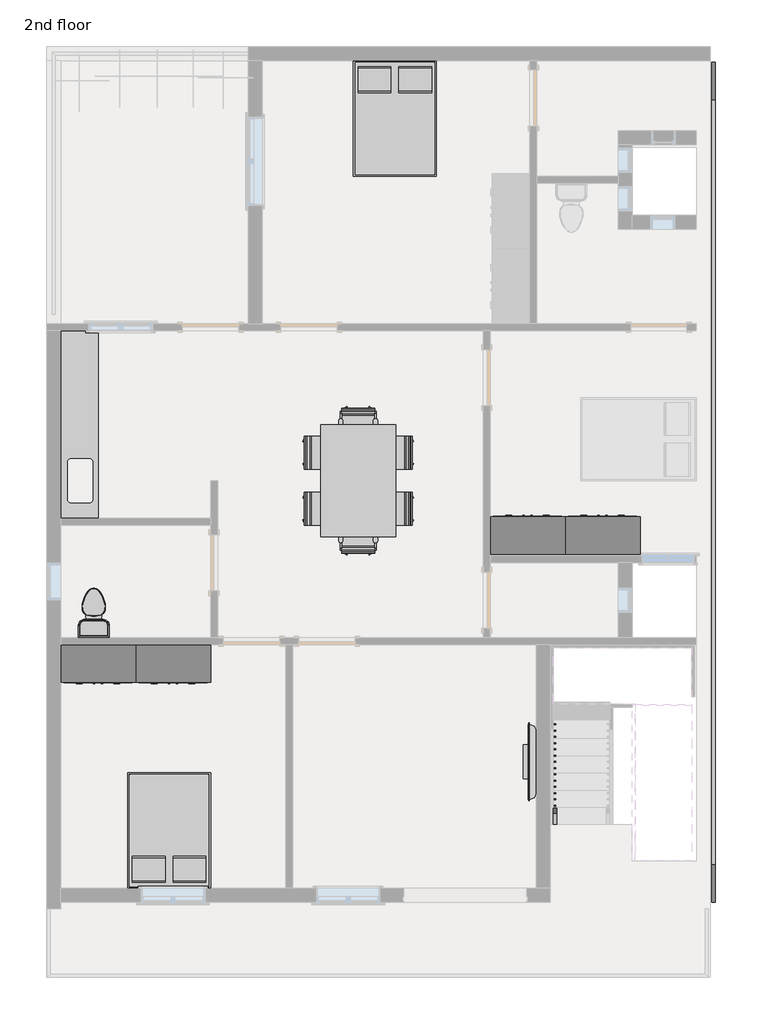
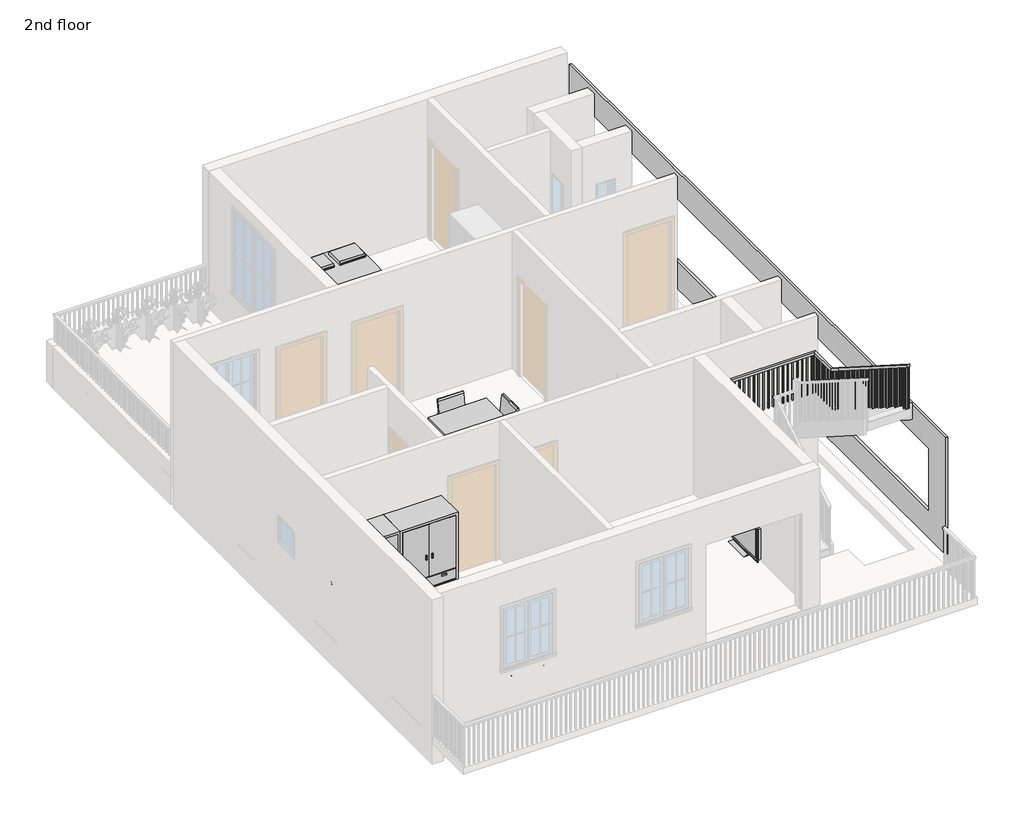
# One storey, part 4 of 5: 16 furniture elements, 1 flow terminal, 1 railing.
"""IFC4 building model written with IfcOpenShell, lengths in millimetres."""

from ifc_helpers import new_model, si_unit, frame, origin, place, context, project, spatial, polyline, outline, extrude, faceted_brep, transform, mapped, element, save
from components import toilet_domestic_3d_toilet_domestic_3d_9ecb9d01, toilet_domestic_3d_toilet_domestic_3d_e67c3c64, furniture_b58f7881, casework_4_casework_4_12d1038f, chair_task_chair_task_b7f3823b, chair_task_arms_chair_task_arms_fa5a08ef, furniture_771c7099, furniture_0b81fedb, furniture_0bcc43ae, furniture_82e269c4

model = new_model("IFC4")

# Units and contexts
model_context = context("Model", 3, world=origin())
ifc_project = project(units=[si_unit("LENGTHUNIT", "METRE", prefix="MILLI")], contexts=[model_context])

# Site, building, storey
site = spatial("IfcSite", under=ifc_project)
building = spatial("IfcBuilding", under=site)
storey = spatial("IfcBuildingStorey", under=building, Name="2nd floor", Elevation=7010.4)

# Flow terminal
placement = place(None, origin())
toilet_domestic_3d_toilet_domestic_3d_shape = toilet_domestic_3d_toilet_domestic_3d_9ecb9d01(model_context)
toilet_domestic_3d_toilet_domestic_3d_2_shape = toilet_domestic_3d_toilet_domestic_3d_e67c3c64(model_context)
element("IfcFlowTerminal", 1, ObjectType="Toilet-Domestic-3D : Toilet-Domestic-3D", at=placement, inside=storey, context=model_context, shape_type="MappedRepresentation", body=[
    mapped(toilet_domestic_3d_toilet_domestic_3d_shape, transform((-7342.9058187, 3694.2738062, 7010.4), x_axis=(1.0, 0.0, 0.0), y_axis=(0.0, 1.0, 0.0), z_axis=(0.0, 0.0, 1.0))),
    mapped(toilet_domestic_3d_toilet_domestic_3d_2_shape, transform((-7342.9058187, 3694.2738062, 7010.4), x_axis=(1.0, 0.0, 0.0), y_axis=(0.0, 1.0, 0.0), z_axis=(0.0, 0.0, 1.0))),
])

# Furniture
furniture_shape = furniture_b58f7881(model_context)
element("IfcFurniture", 2, ObjectType="Bed-Box : Double 53\" x 74\"", at=placement, inside=storey, context=model_context, shape_type="MappedRepresentation", body=[
    mapped(furniture_shape, transform((-2785.3023187, 11872.8553007, 7010.4), x_axis=(1.0, 0.0, 0.0), y_axis=(0.0, 1.0, 0.0), z_axis=(0.0, 0.0, 1.0))),
])
element("IfcFurniture", 3, ObjectType="Bed-Box : Double 53\" x 74\"", at=placement, inside=storey, context=model_context, shape_type="MappedRepresentation", body=[
    mapped(furniture_shape, transform((-5777.2974007, -178.4037157, 7010.4), x_axis=(-1.0, 0.0, 0.0), y_axis=(0.0, -1.0, 0.0), z_axis=(0.0, 0.0, 1.0))),
])
casework_4_casework_4_shape = casework_4_casework_4_12d1038f(model_context)
element("IfcFurniture", 4, ObjectType="Casework 4 : Casework 4", at=placement, inside=storey, context=model_context, shape_type="MappedRepresentation", body=[
    mapped(casework_4_casework_4_shape, transform((0.0, 0.0, 0.0), x_axis=(1.0, 0.0, 0.0), y_axis=(0.0, 1.0, 0.0), z_axis=(0.0, 0.0, 1.0))),
])
chair_task_chair_task_shape = chair_task_chair_task_b7f3823b(model_context)
element("IfcFurniture", 5, ObjectType="Chair-Task : Chair-Task", at=placement, inside=storey, context=model_context, shape_type="MappedRepresentation", body=[
    mapped(chair_task_chair_task_shape, transform((-3671.5957614, 6343.8166122, 7010.4), x_axis=(0.0, -1.0, 0.0), y_axis=(1.0, 0.0, 0.0), z_axis=(0.0, 0.0, 1.0))),
])
element("IfcFurniture", 6, ObjectType="Chair-Task : Chair-Task", at=placement, inside=storey, context=model_context, shape_type="MappedRepresentation", body=[
    mapped(chair_task_chair_task_shape, transform((-2414.5039581, 6061.8349729, 7010.4), x_axis=(0.0, 1.0, 0.0), y_axis=(-1.0, 0.0, 0.0), z_axis=(0.0, 0.0, 1.0))),
])
element("IfcFurniture", 7, ObjectType="Chair-Task : Chair-Task", at=placement, inside=storey, context=model_context, shape_type="MappedRepresentation", body=[
    mapped(chair_task_chair_task_shape, transform((-3671.5957614, 5429.4166122, 7010.4), x_axis=(0.0, -1.0, 0.0), y_axis=(1.0, 0.0, 0.0), z_axis=(0.0, 0.0, 1.0))),
])
element("IfcFurniture", 8, ObjectType="Chair-Task : Chair-Task", at=placement, inside=storey, context=model_context, shape_type="MappedRepresentation", body=[
    mapped(chair_task_chair_task_shape, transform((-2414.5039581, 5147.4349729, 7010.4), x_axis=(0.0, 1.0, 0.0), y_axis=(-1.0, 0.0, 0.0), z_axis=(0.0, 0.0, 1.0))),
])
chair_task_arms_chair_task_arms_shape = chair_task_arms_chair_task_arms_fa5a08ef(model_context)
element("IfcFurniture", 9, ObjectType="Chair-Task Arms : Chair-Task Arms", at=placement, inside=storey, context=model_context, shape_type="MappedRepresentation", body=[
    mapped(chair_task_arms_chair_task_arms_shape, transform((-3184.0406794, 4812.2798909, 7010.4), x_axis=(1.0, 0.0, 0.0), y_axis=(0.0, 1.0, 0.0), z_axis=(0.0, 0.0, 1.0))),
])
element("IfcFurniture", 10, ObjectType="Chair-Task Arms : Chair-Task Arms", at=placement, inside=storey, context=model_context, shape_type="MappedRepresentation", body=[
    mapped(chair_task_arms_chair_task_arms_shape, transform((-2902.05904, 6678.9716942, 7010.4), x_axis=(-1.0, 0.0, 0.0), y_axis=(0.0, -1.0, 0.0), z_axis=(0.0, 0.0, 1.0))),
])
furniture_2_shape = furniture_771c7099(model_context)
element("IfcFurniture", 11, ObjectType="Counter Top w Sink Hole : 24\" Depth", at=placement, inside=storey, context=model_context, shape_type="MappedRepresentation", body=[
    mapped(furniture_2_shape, transform((-7907.1498597, 6336.4880876, 7010.4), x_axis=(0.0, 1.0, 0.0), y_axis=(-1.0, 0.0, 0.0), z_axis=(0.0, 0.0, 1.0))),
])
furniture_3_shape = furniture_0b81fedb(model_context)
element("IfcFurniture", 12, ObjectType="TV - Flat Screen : 50\"", at=placement, inside=storey, context=model_context, shape_type="MappedRepresentation", body=[
    mapped(furniture_3_shape, transform((-205.9884834, 1169.6812784, 7010.4), x_axis=(0.0, -1.0, 0.0), y_axis=(1.0, 0.0, 0.0), z_axis=(0.0, 0.0, 1.0))),
])
furniture_4_shape = furniture_0bcc43ae(model_context)
element("IfcFurniture", 13, ObjectType="Table-Conference2 w Chairs : 48\" x 144\"", at=placement, inside=storey, context=model_context, shape_type="MappedRepresentation", body=[
    mapped(furniture_4_shape, transform((-3043.0498597, 5745.6257925, 7010.4), x_axis=(0.0, 1.0, 0.0), y_axis=(-1.0, 0.0, 0.0), z_axis=(0.0, 0.0, 1.0))),
])
furniture_5_shape = furniture_82e269c4(model_context)
element("IfcFurniture", 14, ObjectType="Wardrobe : 48\" x 72\" x 24\"", at=placement, inside=storey, context=model_context, shape_type="MappedRepresentation", body=[
    mapped(furniture_5_shape, transform((-556.3431196, 4272.886983, 7010.4), x_axis=(-1.0, 0.0, 0.0), y_axis=(0.0, -1.0, 0.0), z_axis=(0.0, 0.0, 1.0))),
])
element("IfcFurniture", 15, ObjectType="Wardrobe : 48\" x 72\" x 24\"", at=placement, inside=storey, context=model_context, shape_type="MappedRepresentation", body=[
    mapped(furniture_5_shape, transform((662.8568804, 4272.886983, 7010.4), x_axis=(-1.0, 0.0, 0.0), y_axis=(0.0, -1.0, 0.0), z_axis=(0.0, 0.0, 1.0))),
])
element("IfcFurniture", 16, ObjectType="Wardrobe : 48\" x 72\" x 24\"", at=placement, inside=storey, context=model_context, shape_type="MappedRepresentation", body=[
    mapped(furniture_5_shape, transform((-7002.9565999, 3357.5646021, 7010.4), x_axis=(1.0, 0.0, 0.0), y_axis=(0.0, 1.0, 0.0), z_axis=(0.0, 0.0, 1.0))),
])
element("IfcFurniture", 17, ObjectType="Wardrobe : 48\" x 72\" x 24\"", at=placement, inside=storey, context=model_context, shape_type="MappedRepresentation", body=[
    mapped(furniture_5_shape, transform((-5783.7565999, 3357.5646021, 7010.4), x_axis=(1.0, 0.0, 0.0), y_axis=(0.0, 1.0, 0.0), z_axis=(0.0, 0.0, 1.0))),
])

# Railing
element("IfcRailing", 18, ObjectType="Handrail - Rectangular", at=placement, inside=storey, context=model_context, shape_type="SolidModel", body=[
    faceted_brep([(131.9501403, 157.6257925, 8102.6), (131.9501403, 157.6257925, 8042.386276), (182.7501403, 157.6257925, 8042.386276), (182.7501403, 157.6257925, 8102.6), (131.9501403, 2113.4257925, 9347.2), (131.9501403, 2128.2187874, 9296.4), (182.7501403, 2128.2187874, 9296.4), (182.7501403, 2113.4257925, 9347.2), (131.9501403, 3027.8257925, 9347.2), (131.9501403, 3027.8257925, 9296.4), (182.7501403, 2977.0257925, 9296.4), (182.7501403, 2977.0257925, 9347.2), (2379.8501403, 3027.8257925, 9347.2), (2379.8501403, 3027.8257925, 9296.4), (2329.0501403, 2977.0257925, 9296.4), (2329.0501403, 2977.0257925, 9347.2), (2379.8501403, 2392.8257925, 9347.2), (2379.8501403, 2378.0327976, 9296.4), (2329.0501403, 2378.0327976, 9296.4), (2329.0501403, 2392.8257925, 9347.2), (2379.8501403, 2113.4257925, 9525.0), (2379.8501403, 2086.1525175, 9482.1419964), (2329.0501403, 2086.1525175, 9482.1419964), (2329.0501403, 2113.4257925, 9525.0), (2379.8501403, -401.1742075, 11125.2), (2329.0501403, -401.1742075, 11125.2), (2329.0501403, -401.1742075, 11064.986276), (2379.8501403, -401.1742075, 11064.986276)], [[[0, 1, 2, 3]], [[1, 0, 4, 5]], [[2, 1, 5, 6]], [[3, 2, 6, 7]], [[0, 3, 7, 4]], [[5, 4, 8, 9]], [[6, 5, 9, 10]], [[7, 6, 10, 11]], [[4, 7, 11, 8]], [[9, 8, 12, 13]], [[10, 9, 13, 14]], [[11, 10, 14, 15]], [[8, 11, 15, 12]], [[13, 12, 16, 17]], [[14, 13, 17, 18]], [[15, 14, 18, 19]], [[12, 15, 19, 16]], [[17, 16, 20, 21]], [[18, 17, 21, 22]], [[19, 18, 22, 23]], [[16, 19, 23, 20]], [[24, 25, 26, 27]], [[21, 20, 24, 27]], [[22, 21, 27, 26]], [[23, 22, 26, 25]], [[20, 23, 25, 24]]]),
    extrude(outline(polyline([(-315.4492075, 11010.4340032), (-315.4492075, 10033.0), (-334.4992075, 10033.0), (-334.4992075, 11022.5567305), (-315.4492075, 11010.4340032)])), frame((2344.9251403, 0.0, 0.0), z_axis=(1.0, 0.0, 0.0), x_axis=(0.0, 1.0, 0.0)), (0.0, 0.0, 1.0), 19.05),
    extrude(outline(polyline([(-213.8492075, 10945.7794578), (-213.8492075, 10033.0), (-232.8992075, 10033.0), (-232.8992075, 10957.9021851), (-213.8492075, 10945.7794578)])), frame((2344.9251403, 0.0, 0.0), z_axis=(1.0, 0.0, 0.0), x_axis=(0.0, 1.0, 0.0)), (0.0, 0.0, 1.0), 19.05),
    extrude(outline(polyline([(-112.2492075, 10881.1249123), (-112.2492075, 10033.0), (-131.2992075, 10033.0), (-131.2992075, 10893.2476396), (-112.2492075, 10881.1249123)])), frame((2344.9251403, 0.0, 0.0), z_axis=(1.0, 0.0, 0.0), x_axis=(0.0, 1.0, 0.0)), (0.0, 0.0, 1.0), 19.05),
    extrude(outline(polyline([(-10.6492075, 10816.4703669), (-10.6492075, 9855.2), (-29.6992075, 9855.2), (-29.6992075, 10828.5930941), (-10.6492075, 10816.4703669)])), frame((2344.9251403, 0.0, 0.0), z_axis=(1.0, 0.0, 0.0), x_axis=(0.0, 1.0, 0.0)), (0.0, 0.0, 1.0), 19.05),
    extrude(outline(polyline([(90.9507925, 10751.8158214), (90.9507925, 9855.2), (71.9007925, 9855.2), (71.9007925, 10763.9385487), (90.9507925, 10751.8158214)])), frame((2344.9251403, 0.0, 0.0), z_axis=(1.0, 0.0, 0.0), x_axis=(0.0, 1.0, 0.0)), (0.0, 0.0, 1.0), 19.05),
    extrude(outline(polyline([(192.5507925, 10687.161276), (192.5507925, 9677.4), (173.5007925, 9677.4), (173.5007925, 10699.2840032), (192.5507925, 10687.161276)])), frame((2344.9251403, 0.0, 0.0), z_axis=(1.0, 0.0, 0.0), x_axis=(0.0, 1.0, 0.0)), (0.0, 0.0, 1.0), 19.05),
    extrude(outline(polyline([(294.1507925, 10622.5067305), (294.1507925, 9677.4), (275.1007925, 9677.4), (275.1007925, 10634.6294578), (294.1507925, 10622.5067305)])), frame((2344.9251403, 0.0, 0.0), z_axis=(1.0, 0.0, 0.0), x_axis=(0.0, 1.0, 0.0)), (0.0, 0.0, 1.0), 19.05),
    extrude(outline(polyline([(395.7507925, 10557.8521851), (395.7507925, 9677.4), (376.7007925, 9677.4), (376.7007925, 10569.9749123), (395.7507925, 10557.8521851)])), frame((2344.9251403, 0.0, 0.0), z_axis=(1.0, 0.0, 0.0), x_axis=(0.0, 1.0, 0.0)), (0.0, 0.0, 1.0), 19.05),
    extrude(outline(polyline([(497.3507925, 10493.1976396), (497.3507925, 9499.6), (478.3007925, 9499.6), (478.3007925, 10505.3203669), (497.3507925, 10493.1976396)])), frame((2344.9251403, 0.0, 0.0), z_axis=(1.0, 0.0, 0.0), x_axis=(0.0, 1.0, 0.0)), (0.0, 0.0, 1.0), 19.05),
    extrude(outline(polyline([(598.9507925, 10428.5430941), (598.9507925, 9499.6), (579.9007925, 9499.6), (579.9007925, 10440.6658214), (598.9507925, 10428.5430941)])), frame((2344.9251403, 0.0, 0.0), z_axis=(1.0, 0.0, 0.0), x_axis=(0.0, 1.0, 0.0)), (0.0, 0.0, 1.0), 19.05),
    extrude(outline(polyline([(700.5507925, 10363.8885487), (700.5507925, 9499.6), (681.5007925, 9499.6), (681.5007925, 10376.011276), (700.5507925, 10363.8885487)])), frame((2344.9251403, 0.0, 0.0), z_axis=(1.0, 0.0, 0.0), x_axis=(0.0, 1.0, 0.0)), (0.0, 0.0, 1.0), 19.05),
    extrude(outline(polyline([(802.1507925, 10299.2340032), (802.1507925, 9321.8), (783.1007925, 9321.8), (783.1007925, 10311.3567305), (802.1507925, 10299.2340032)])), frame((2344.9251403, 0.0, 0.0), z_axis=(1.0, 0.0, 0.0), x_axis=(0.0, 1.0, 0.0)), (0.0, 0.0, 1.0), 19.05),
    extrude(outline(polyline([(903.7507925, 10234.5794578), (903.7507925, 9321.8), (884.7007925, 9321.8), (884.7007925, 10246.7021851), (903.7507925, 10234.5794578)])), frame((2344.9251403, 0.0, 0.0), z_axis=(1.0, 0.0, 0.0), x_axis=(0.0, 1.0, 0.0)), (0.0, 0.0, 1.0), 19.05),
    extrude(outline(polyline([(1005.3507925, 10169.9249123), (1005.3507925, 9321.8), (986.3007925, 9321.8), (986.3007925, 10182.0476396), (1005.3507925, 10169.9249123)])), frame((2344.9251403, 0.0, 0.0), z_axis=(1.0, 0.0, 0.0), x_axis=(0.0, 1.0, 0.0)), (0.0, 0.0, 1.0), 19.05),
    extrude(outline(polyline([(1106.9507925, 10105.2703669), (1106.9507925, 9144.0), (1087.9007925, 9144.0), (1087.9007925, 10117.3930941), (1106.9507925, 10105.2703669)])), frame((2344.9251403, 0.0, 0.0), z_axis=(1.0, 0.0, 0.0), x_axis=(0.0, 1.0, 0.0)), (0.0, 0.0, 1.0), 19.05),
    extrude(outline(polyline([(1208.5507925, 10040.6158214), (1208.5507925, 9144.0), (1189.5007925, 9144.0), (1189.5007925, 10052.7385487), (1208.5507925, 10040.6158214)])), frame((2344.9251403, 0.0, 0.0), z_axis=(1.0, 0.0, 0.0), x_axis=(0.0, 1.0, 0.0)), (0.0, 0.0, 1.0), 19.05),
    extrude(outline(polyline([(1310.1507925, 9975.961276), (1310.1507925, 8966.2), (1291.1007925, 8966.2), (1291.1007925, 9988.0840032), (1310.1507925, 9975.961276)])), frame((2344.9251403, 0.0, 0.0), z_axis=(1.0, 0.0, 0.0), x_axis=(0.0, 1.0, 0.0)), (0.0, 0.0, 1.0), 19.05),
    extrude(outline(polyline([(1411.7507925, 9911.3067305), (1411.7507925, 8966.2), (1392.7007925, 8966.2), (1392.7007925, 9923.4294578), (1411.7507925, 9911.3067305)])), frame((2344.9251403, 0.0, 0.0), z_axis=(1.0, 0.0, 0.0), x_axis=(0.0, 1.0, 0.0)), (0.0, 0.0, 1.0), 19.05),
    extrude(outline(polyline([(1513.3507925, 9846.6521851), (1513.3507925, 8966.2), (1494.3007925, 8966.2), (1494.3007925, 9858.7749123), (1513.3507925, 9846.6521851)])), frame((2344.9251403, 0.0, 0.0), z_axis=(1.0, 0.0, 0.0), x_axis=(0.0, 1.0, 0.0)), (0.0, 0.0, 1.0), 19.05),
    extrude(outline(polyline([(1614.9507925, 9781.9976396), (1614.9507925, 8788.4), (1595.9007925, 8788.4), (1595.9007925, 9794.1203669), (1614.9507925, 9781.9976396)])), frame((2344.9251403, 0.0, 0.0), z_axis=(1.0, 0.0, 0.0), x_axis=(0.0, 1.0, 0.0)), (0.0, 0.0, 1.0), 19.05),
    extrude(outline(polyline([(1716.5507925, 9717.3430941), (1716.5507925, 8788.4), (1697.5007925, 8788.4), (1697.5007925, 9729.4658214), (1716.5507925, 9717.3430941)])), frame((2344.9251403, 0.0, 0.0), z_axis=(1.0, 0.0, 0.0), x_axis=(0.0, 1.0, 0.0)), (0.0, 0.0, 1.0), 19.05),
    extrude(outline(polyline([(1818.1507925, 9652.6885487), (1818.1507925, 8788.4), (1799.1007925, 8788.4), (1799.1007925, 9664.811276), (1818.1507925, 9652.6885487)])), frame((2344.9251403, 0.0, 0.0), z_axis=(1.0, 0.0, 0.0), x_axis=(0.0, 1.0, 0.0)), (0.0, 0.0, 1.0), 19.05),
    extrude(outline(polyline([(1919.7507925, 9588.0340032), (1919.7507925, 8610.6), (1900.7007925, 8610.6), (1900.7007925, 9600.1567305), (1919.7507925, 9588.0340032)])), frame((2344.9251403, 0.0, 0.0), z_axis=(1.0, 0.0, 0.0), x_axis=(0.0, 1.0, 0.0)), (0.0, 0.0, 1.0), 19.05),
    extrude(outline(polyline([(2021.3507925, 9523.3794578), (2021.3507925, 8610.6), (2002.3007925, 8610.6), (2002.3007925, 9535.5021851), (2021.3507925, 9523.3794578)])), frame((2344.9251403, 0.0, 0.0), z_axis=(1.0, 0.0, 0.0), x_axis=(0.0, 1.0, 0.0)), (0.0, 0.0, 1.0), 19.05),
    extrude(outline(polyline([(2199.1507925, 9410.2340032), (2199.1507925, 8432.8), (2180.1007925, 8432.8), (2180.1007925, 9422.3567305), (2199.1507925, 9410.2340032)])), frame((2344.9251403, 0.0, 0.0), z_axis=(1.0, 0.0, 0.0), x_axis=(0.0, 1.0, 0.0)), (0.0, 0.0, 1.0), 19.05),
    extrude(outline(polyline([(2300.7507925, 9345.5794578), (2300.7507925, 8432.8), (2281.7007925, 8432.8), (2281.7007925, 9357.7021851), (2300.7507925, 9345.5794578)])), frame((2344.9251403, 0.0, 0.0), z_axis=(1.0, 0.0, 0.0), x_axis=(0.0, 1.0, 0.0)), (0.0, 0.0, 1.0), 19.05),
    extrude(outline(polyline([(2363.9751403, 2402.3507925), (2363.9751403, 2383.3007925), (2344.9251403, 2383.3007925), (2344.9251403, 2402.3507925), (2363.9751403, 2402.3507925)])), frame((0.0, 0.0, 8432.8), z_axis=(0.0, 0.0, 1.0), x_axis=(1.0, 0.0, 0.0)), (0.0, 0.0, 1.0), 863.6),
    extrude(outline(polyline([(2363.9751403, 2503.9507925), (2363.9751403, 2484.9007925), (2344.9251403, 2484.9007925), (2344.9251403, 2503.9507925), (2363.9751403, 2503.9507925)])), frame((0.0, 0.0, 8432.8), z_axis=(0.0, 0.0, 1.0), x_axis=(1.0, 0.0, 0.0)), (0.0, 0.0, 1.0), 863.6),
    extrude(outline(polyline([(2363.9751403, 2605.5507925), (2363.9751403, 2586.5007925), (2344.9251403, 2586.5007925), (2344.9251403, 2605.5507925), (2363.9751403, 2605.5507925)])), frame((0.0, 0.0, 8432.8), z_axis=(0.0, 0.0, 1.0), x_axis=(1.0, 0.0, 0.0)), (0.0, 0.0, 1.0), 863.6),
    extrude(outline(polyline([(2363.9751403, 2707.1507925), (2363.9751403, 2688.1007925), (2344.9251403, 2688.1007925), (2344.9251403, 2707.1507925), (2363.9751403, 2707.1507925)])), frame((0.0, 0.0, 8432.8), z_axis=(0.0, 0.0, 1.0), x_axis=(1.0, 0.0, 0.0)), (0.0, 0.0, 1.0), 863.6),
    extrude(outline(polyline([(2363.9751403, 2808.7507925), (2363.9751403, 2789.7007925), (2344.9251403, 2789.7007925), (2344.9251403, 2808.7507925), (2363.9751403, 2808.7507925)])), frame((0.0, 0.0, 8432.8), z_axis=(0.0, 0.0, 1.0), x_axis=(1.0, 0.0, 0.0)), (0.0, 0.0, 1.0), 863.6),
    extrude(outline(polyline([(2363.9751403, 2910.3507925), (2363.9751403, 2891.3007925), (2344.9251403, 2891.3007925), (2344.9251403, 2910.3507925), (2363.9751403, 2910.3507925)])), frame((0.0, 0.0, 8432.8), z_axis=(0.0, 0.0, 1.0), x_axis=(1.0, 0.0, 0.0)), (0.0, 0.0, 1.0), 863.6),
    extrude(outline(polyline([(2281.4251403, 3011.9507925), (2300.4751403, 3011.9507925), (2300.4751403, 2992.9007925), (2281.4251403, 2992.9007925), (2281.4251403, 3011.9507925)])), frame((0.0, 0.0, 8432.8), z_axis=(0.0, 0.0, 1.0), x_axis=(1.0, 0.0, 0.0)), (0.0, 0.0, 1.0), 863.6),
    extrude(outline(polyline([(2179.8251403, 3011.9507925), (2198.8751403, 3011.9507925), (2198.8751403, 2992.9007925), (2179.8251403, 2992.9007925), (2179.8251403, 3011.9507925)])), frame((0.0, 0.0, 8432.8), z_axis=(0.0, 0.0, 1.0), x_axis=(1.0, 0.0, 0.0)), (0.0, 0.0, 1.0), 863.6),
    extrude(outline(polyline([(2078.2251403, 3011.9507925), (2097.2751403, 3011.9507925), (2097.2751403, 2992.9007925), (2078.2251403, 2992.9007925), (2078.2251403, 3011.9507925)])), frame((0.0, 0.0, 8432.8), z_axis=(0.0, 0.0, 1.0), x_axis=(1.0, 0.0, 0.0)), (0.0, 0.0, 1.0), 863.6),
    extrude(outline(polyline([(1976.6251403, 3011.9507925), (1995.6751403, 3011.9507925), (1995.6751403, 2992.9007925), (1976.6251403, 2992.9007925), (1976.6251403, 3011.9507925)])), frame((0.0, 0.0, 8432.8), z_axis=(0.0, 0.0, 1.0), x_axis=(1.0, 0.0, 0.0)), (0.0, 0.0, 1.0), 863.6),
    extrude(outline(polyline([(1875.0251403, 3011.9507925), (1894.0751403, 3011.9507925), (1894.0751403, 2992.9007925), (1875.0251403, 2992.9007925), (1875.0251403, 3011.9507925)])), frame((0.0, 0.0, 8432.8), z_axis=(0.0, 0.0, 1.0), x_axis=(1.0, 0.0, 0.0)), (0.0, 0.0, 1.0), 863.6),
    extrude(outline(polyline([(1773.4251403, 3011.9507925), (1792.4751403, 3011.9507925), (1792.4751403, 2992.9007925), (1773.4251403, 2992.9007925), (1773.4251403, 3011.9507925)])), frame((0.0, 0.0, 8432.8), z_axis=(0.0, 0.0, 1.0), x_axis=(1.0, 0.0, 0.0)), (0.0, 0.0, 1.0), 863.6),
    extrude(outline(polyline([(1671.8251403, 3011.9507925), (1690.8751403, 3011.9507925), (1690.8751403, 2992.9007925), (1671.8251403, 2992.9007925), (1671.8251403, 3011.9507925)])), frame((0.0, 0.0, 8432.8), z_axis=(0.0, 0.0, 1.0), x_axis=(1.0, 0.0, 0.0)), (0.0, 0.0, 1.0), 863.6),
    extrude(outline(polyline([(1570.2251403, 3011.9507925), (1589.2751403, 3011.9507925), (1589.2751403, 2992.9007925), (1570.2251403, 2992.9007925), (1570.2251403, 3011.9507925)])), frame((0.0, 0.0, 8432.8), z_axis=(0.0, 0.0, 1.0), x_axis=(1.0, 0.0, 0.0)), (0.0, 0.0, 1.0), 863.6),
    extrude(outline(polyline([(1468.6251403, 3011.9507925), (1487.6751403, 3011.9507925), (1487.6751403, 2992.9007925), (1468.6251403, 2992.9007925), (1468.6251403, 3011.9507925)])), frame((0.0, 0.0, 8432.8), z_axis=(0.0, 0.0, 1.0), x_axis=(1.0, 0.0, 0.0)), (0.0, 0.0, 1.0), 863.6),
    extrude(outline(polyline([(1367.0251403, 3011.9507925), (1386.0751403, 3011.9507925), (1386.0751403, 2992.9007925), (1367.0251403, 2992.9007925), (1367.0251403, 3011.9507925)])), frame((0.0, 0.0, 8432.8), z_axis=(0.0, 0.0, 1.0), x_axis=(1.0, 0.0, 0.0)), (0.0, 0.0, 1.0), 863.6),
    extrude(outline(polyline([(1265.4251403, 3011.9507925), (1284.4751403, 3011.9507925), (1284.4751403, 2992.9007925), (1265.4251403, 2992.9007925), (1265.4251403, 3011.9507925)])), frame((0.0, 0.0, 8432.8), z_axis=(0.0, 0.0, 1.0), x_axis=(1.0, 0.0, 0.0)), (0.0, 0.0, 1.0), 863.6),
    extrude(outline(polyline([(1163.8251403, 3011.9507925), (1182.8751403, 3011.9507925), (1182.8751403, 2992.9007925), (1163.8251403, 2992.9007925), (1163.8251403, 3011.9507925)])), frame((0.0, 0.0, 8432.8), z_axis=(0.0, 0.0, 1.0), x_axis=(1.0, 0.0, 0.0)), (0.0, 0.0, 1.0), 863.6),
    extrude(outline(polyline([(1062.2251403, 3011.9507925), (1081.2751403, 3011.9507925), (1081.2751403, 2992.9007925), (1062.2251403, 2992.9007925), (1062.2251403, 3011.9507925)])), frame((0.0, 0.0, 8432.8), z_axis=(0.0, 0.0, 1.0), x_axis=(1.0, 0.0, 0.0)), (0.0, 0.0, 1.0), 863.6),
    extrude(outline(polyline([(960.6251403, 3011.9507925), (979.6751403, 3011.9507925), (979.6751403, 2992.9007925), (960.6251403, 2992.9007925), (960.6251403, 3011.9507925)])), frame((0.0, 0.0, 8432.8), z_axis=(0.0, 0.0, 1.0), x_axis=(1.0, 0.0, 0.0)), (0.0, 0.0, 1.0), 863.6),
    extrude(outline(polyline([(859.0251403, 3011.9507925), (878.0751403, 3011.9507925), (878.0751403, 2992.9007925), (859.0251403, 2992.9007925), (859.0251403, 3011.9507925)])), frame((0.0, 0.0, 8432.8), z_axis=(0.0, 0.0, 1.0), x_axis=(1.0, 0.0, 0.0)), (0.0, 0.0, 1.0), 863.6),
    extrude(outline(polyline([(757.4251403, 3011.9507925), (776.4751403, 3011.9507925), (776.4751403, 2992.9007925), (757.4251403, 2992.9007925), (757.4251403, 3011.9507925)])), frame((0.0, 0.0, 8432.8), z_axis=(0.0, 0.0, 1.0), x_axis=(1.0, 0.0, 0.0)), (0.0, 0.0, 1.0), 863.6),
    extrude(outline(polyline([(655.8251403, 3011.9507925), (674.8751403, 3011.9507925), (674.8751403, 2992.9007925), (655.8251403, 2992.9007925), (655.8251403, 3011.9507925)])), frame((0.0, 0.0, 8432.8), z_axis=(0.0, 0.0, 1.0), x_axis=(1.0, 0.0, 0.0)), (0.0, 0.0, 1.0), 863.6),
    extrude(outline(polyline([(554.2251403, 3011.9507925), (573.2751403, 3011.9507925), (573.2751403, 2992.9007925), (554.2251403, 2992.9007925), (554.2251403, 3011.9507925)])), frame((0.0, 0.0, 8432.8), z_axis=(0.0, 0.0, 1.0), x_axis=(1.0, 0.0, 0.0)), (0.0, 0.0, 1.0), 863.6),
    extrude(outline(polyline([(452.6251403, 3011.9507925), (471.6751403, 3011.9507925), (471.6751403, 2992.9007925), (452.6251403, 2992.9007925), (452.6251403, 3011.9507925)])), frame((0.0, 0.0, 8432.8), z_axis=(0.0, 0.0, 1.0), x_axis=(1.0, 0.0, 0.0)), (0.0, 0.0, 1.0), 863.6),
    extrude(outline(polyline([(351.0251403, 3011.9507925), (370.0751403, 3011.9507925), (370.0751403, 2992.9007925), (351.0251403, 2992.9007925), (351.0251403, 3011.9507925)])), frame((0.0, 0.0, 8432.8), z_axis=(0.0, 0.0, 1.0), x_axis=(1.0, 0.0, 0.0)), (0.0, 0.0, 1.0), 863.6),
    extrude(outline(polyline([(249.4251403, 3011.9507925), (268.4751403, 3011.9507925), (268.4751403, 2992.9007925), (249.4251403, 2992.9007925), (249.4251403, 3011.9507925)])), frame((0.0, 0.0, 8432.8), z_axis=(0.0, 0.0, 1.0), x_axis=(1.0, 0.0, 0.0)), (0.0, 0.0, 1.0), 863.6),
    extrude(outline(polyline([(147.8251403, 2916.7007925), (147.8251403, 2935.7507925), (166.8751403, 2935.7507925), (166.8751403, 2916.7007925), (147.8251403, 2916.7007925)])), frame((0.0, 0.0, 8432.8), z_axis=(0.0, 0.0, 1.0), x_axis=(1.0, 0.0, 0.0)), (0.0, 0.0, 1.0), 863.6),
    extrude(outline(polyline([(147.8251403, 2815.1007925), (147.8251403, 2834.1507925), (166.8751403, 2834.1507925), (166.8751403, 2815.1007925), (147.8251403, 2815.1007925)])), frame((0.0, 0.0, 8432.8), z_axis=(0.0, 0.0, 1.0), x_axis=(1.0, 0.0, 0.0)), (0.0, 0.0, 1.0), 863.6),
    extrude(outline(polyline([(147.8251403, 2713.5007925), (147.8251403, 2732.5507925), (166.8751403, 2732.5507925), (166.8751403, 2713.5007925), (147.8251403, 2713.5007925)])), frame((0.0, 0.0, 8432.8), z_axis=(0.0, 0.0, 1.0), x_axis=(1.0, 0.0, 0.0)), (0.0, 0.0, 1.0), 863.6),
    extrude(outline(polyline([(147.8251403, 2611.9007925), (147.8251403, 2630.9507925), (166.8751403, 2630.9507925), (166.8751403, 2611.9007925), (147.8251403, 2611.9007925)])), frame((0.0, 0.0, 8432.8), z_axis=(0.0, 0.0, 1.0), x_axis=(1.0, 0.0, 0.0)), (0.0, 0.0, 1.0), 863.6),
    extrude(outline(polyline([(147.8251403, 2510.3007925), (147.8251403, 2529.3507925), (166.8751403, 2529.3507925), (166.8751403, 2510.3007925), (147.8251403, 2510.3007925)])), frame((0.0, 0.0, 8432.8), z_axis=(0.0, 0.0, 1.0), x_axis=(1.0, 0.0, 0.0)), (0.0, 0.0, 1.0), 863.6),
    extrude(outline(polyline([(147.8251403, 2408.7007925), (147.8251403, 2427.7507925), (166.8751403, 2427.7507925), (166.8751403, 2408.7007925), (147.8251403, 2408.7007925)])), frame((0.0, 0.0, 8432.8), z_axis=(0.0, 0.0, 1.0), x_axis=(1.0, 0.0, 0.0)), (0.0, 0.0, 1.0), 863.6),
    extrude(outline(polyline([(147.8251403, 2307.1007925), (147.8251403, 2326.1507925), (166.8751403, 2326.1507925), (166.8751403, 2307.1007925), (147.8251403, 2307.1007925)])), frame((0.0, 0.0, 8432.8), z_axis=(0.0, 0.0, 1.0), x_axis=(1.0, 0.0, 0.0)), (0.0, 0.0, 1.0), 863.6),
    extrude(outline(polyline([(147.8251403, 2205.5007925), (147.8251403, 2224.5507925), (166.8751403, 2224.5507925), (166.8751403, 2205.5007925), (147.8251403, 2205.5007925)])), frame((0.0, 0.0, 8432.8), z_axis=(0.0, 0.0, 1.0), x_axis=(1.0, 0.0, 0.0)), (0.0, 0.0, 1.0), 863.6),
    extrude(outline(polyline([(2097.5507925, 9276.8840032), (2097.5507925, 8255.0), (2078.5007925, 8255.0), (2078.5007925, 9264.761276), (2097.5507925, 9276.8840032)])), frame((147.8251403, 0.0, 0.0), z_axis=(1.0, 0.0, 0.0), x_axis=(0.0, 1.0, 0.0)), (0.0, 0.0, 1.0), 19.05),
    extrude(outline(polyline([(1995.9507925, 9212.2294578), (1995.9507925, 8255.0), (1976.9007925, 8255.0), (1976.9007925, 9200.1067305), (1995.9507925, 9212.2294578)])), frame((147.8251403, 0.0, 0.0), z_axis=(1.0, 0.0, 0.0), x_axis=(0.0, 1.0, 0.0)), (0.0, 0.0, 1.0), 19.05),
    extrude(outline(polyline([(1894.3507925, 9147.5749123), (1894.3507925, 8255.0), (1875.3007925, 8255.0), (1875.3007925, 9135.4521851), (1894.3507925, 9147.5749123)])), frame((147.8251403, 0.0, 0.0), z_axis=(1.0, 0.0, 0.0), x_axis=(0.0, 1.0, 0.0)), (0.0, 0.0, 1.0), 19.05),
    extrude(outline(polyline([(1792.7507925, 9082.9203669), (1792.7507925, 8077.2), (1773.7007925, 8077.2), (1773.7007925, 9070.7976396), (1792.7507925, 9082.9203669)])), frame((147.8251403, 0.0, 0.0), z_axis=(1.0, 0.0, 0.0), x_axis=(0.0, 1.0, 0.0)), (0.0, 0.0, 1.0), 19.05),
    extrude(outline(polyline([(1691.1507925, 9018.2658214), (1691.1507925, 8077.2), (1672.1007925, 8077.2), (1672.1007925, 9006.1430941), (1691.1507925, 9018.2658214)])), frame((147.8251403, 0.0, 0.0), z_axis=(1.0, 0.0, 0.0), x_axis=(0.0, 1.0, 0.0)), (0.0, 0.0, 1.0), 19.05),
    extrude(outline(polyline([(1589.5507925, 8953.611276), (1589.5507925, 8077.2), (1570.5007925, 8077.2), (1570.5007925, 8941.4885487), (1589.5507925, 8953.611276)])), frame((147.8251403, 0.0, 0.0), z_axis=(1.0, 0.0, 0.0), x_axis=(0.0, 1.0, 0.0)), (0.0, 0.0, 1.0), 19.05),
    extrude(outline(polyline([(1487.9507925, 8888.9567305), (1487.9507925, 7899.4), (1468.9007925, 7899.4), (1468.9007925, 8876.8340032), (1487.9507925, 8888.9567305)])), frame((147.8251403, 0.0, 0.0), z_axis=(1.0, 0.0, 0.0), x_axis=(0.0, 1.0, 0.0)), (0.0, 0.0, 1.0), 19.05),
    extrude(outline(polyline([(1386.3507925, 8824.3021851), (1386.3507925, 7899.4), (1367.3007925, 7899.4), (1367.3007925, 8812.1794578), (1386.3507925, 8824.3021851)])), frame((147.8251403, 0.0, 0.0), z_axis=(1.0, 0.0, 0.0), x_axis=(0.0, 1.0, 0.0)), (0.0, 0.0, 1.0), 19.05),
    extrude(outline(polyline([(1284.7507925, 8759.6476396), (1284.7507925, 7899.4), (1265.7007925, 7899.4), (1265.7007925, 8747.5249123), (1284.7507925, 8759.6476396)])), frame((147.8251403, 0.0, 0.0), z_axis=(1.0, 0.0, 0.0), x_axis=(0.0, 1.0, 0.0)), (0.0, 0.0, 1.0), 19.05),
    extrude(outline(polyline([(1183.1507925, 8694.9930941), (1183.1507925, 7721.6), (1164.1007925, 7721.6), (1164.1007925, 8682.8703669), (1183.1507925, 8694.9930941)])), frame((147.8251403, 0.0, 0.0), z_axis=(1.0, 0.0, 0.0), x_axis=(0.0, 1.0, 0.0)), (0.0, 0.0, 1.0), 19.05),
    extrude(outline(polyline([(1081.5507925, 8630.3385487), (1081.5507925, 7721.6), (1062.5007925, 7721.6), (1062.5007925, 8618.2158214), (1081.5507925, 8630.3385487)])), frame((147.8251403, 0.0, 0.0), z_axis=(1.0, 0.0, 0.0), x_axis=(0.0, 1.0, 0.0)), (0.0, 0.0, 1.0), 19.05),
    extrude(outline(polyline([(979.9507925, 8565.6840032), (979.9507925, 7543.8), (960.9007925, 7543.8), (960.9007925, 8553.561276), (979.9507925, 8565.6840032)])), frame((147.8251403, 0.0, 0.0), z_axis=(1.0, 0.0, 0.0), x_axis=(0.0, 1.0, 0.0)), (0.0, 0.0, 1.0), 19.05),
    extrude(outline(polyline([(878.3507925, 8501.0294578), (878.3507925, 7543.8), (859.3007925, 7543.8), (859.3007925, 8488.9067305), (878.3507925, 8501.0294578)])), frame((147.8251403, 0.0, 0.0), z_axis=(1.0, 0.0, 0.0), x_axis=(0.0, 1.0, 0.0)), (0.0, 0.0, 1.0), 19.05),
    extrude(outline(polyline([(776.7507925, 8436.3749123), (776.7507925, 7543.8), (757.7007925, 7543.8), (757.7007925, 8424.2521851), (776.7507925, 8436.3749123)])), frame((147.8251403, 0.0, 0.0), z_axis=(1.0, 0.0, 0.0), x_axis=(0.0, 1.0, 0.0)), (0.0, 0.0, 1.0), 19.05),
    extrude(outline(polyline([(675.1507925, 8371.7203669), (675.1507925, 7366.0), (656.1007925, 7366.0), (656.1007925, 8359.5976396), (675.1507925, 8371.7203669)])), frame((147.8251403, 0.0, 0.0), z_axis=(1.0, 0.0, 0.0), x_axis=(0.0, 1.0, 0.0)), (0.0, 0.0, 1.0), 19.05),
    extrude(outline(polyline([(573.5507925, 8307.0658214), (573.5507925, 7366.0), (554.5007925, 7366.0), (554.5007925, 8294.9430941), (573.5507925, 8307.0658214)])), frame((147.8251403, 0.0, 0.0), z_axis=(1.0, 0.0, 0.0), x_axis=(0.0, 1.0, 0.0)), (0.0, 0.0, 1.0), 19.05),
    extrude(outline(polyline([(471.9507925, 8242.411276), (471.9507925, 7366.0), (452.9007925, 7366.0), (452.9007925, 8230.2885487), (471.9507925, 8242.411276)])), frame((147.8251403, 0.0, 0.0), z_axis=(1.0, 0.0, 0.0), x_axis=(0.0, 1.0, 0.0)), (0.0, 0.0, 1.0), 19.05),
    extrude(outline(polyline([(370.3507925, 8177.7567305), (370.3507925, 7188.2), (351.3007925, 7188.2), (351.3007925, 8165.6340032), (370.3507925, 8177.7567305)])), frame((147.8251403, 0.0, 0.0), z_axis=(1.0, 0.0, 0.0), x_axis=(0.0, 1.0, 0.0)), (0.0, 0.0, 1.0), 19.05),
    extrude(outline(polyline([(268.7507925, 8113.1021851), (268.7507925, 7188.2), (249.7007925, 7188.2), (249.7007925, 8100.9794578), (268.7507925, 8113.1021851)])), frame((147.8251403, 0.0, 0.0), z_axis=(1.0, 0.0, 0.0), x_axis=(0.0, 1.0, 0.0)), (0.0, 0.0, 1.0), 19.05),
    extrude(outline(polyline([(2122.9507925, 9458.7249123), (2122.9507925, 8432.8), (2103.9007925, 8432.8), (2103.9007925, 9470.8476396), (2122.9507925, 9458.7249123)])), frame((2344.9251403, 0.0, 0.0), z_axis=(1.0, 0.0, 0.0), x_axis=(0.0, 1.0, 0.0)), (0.0, 0.0, 1.0), 19.05),
    extrude(outline(polyline([(2344.9251403, 3011.9507925), (2363.9751403, 3011.9507925), (2363.9751403, 2992.9007925), (2344.9251403, 2992.9007925), (2344.9251403, 3011.9507925)])), frame((0.0, 0.0, 8432.8), z_axis=(0.0, 0.0, 1.0), x_axis=(1.0, 0.0, 0.0)), (0.0, 0.0, 1.0), 863.6),
    extrude(outline(polyline([(147.8251403, 2992.9007925), (147.8251403, 3011.9507925), (166.8751403, 3011.9507925), (166.8751403, 2992.9007925), (147.8251403, 2992.9007925)])), frame((0.0, 0.0, 8432.8), z_axis=(0.0, 0.0, 1.0), x_axis=(1.0, 0.0, 0.0)), (0.0, 0.0, 1.0), 863.6),
    extrude(outline(polyline([(2122.9507925, 9293.0476396), (2122.9507925, 8432.8), (2103.9007925, 8432.8), (2103.9007925, 9280.9249123), (2122.9507925, 9293.0476396)])), frame((147.8251403, 0.0, 0.0), z_axis=(1.0, 0.0, 0.0), x_axis=(0.0, 1.0, 0.0)), (0.0, 0.0, 1.0), 19.05),
    extrude(outline(polyline([(-382.1242075, 11052.8635487), (-382.1242075, 10033.0), (-401.1742075, 10033.0), (-401.1742075, 11064.986276), (-382.1242075, 11052.8635487)])), frame((2344.9251403, 0.0, 0.0), z_axis=(1.0, 0.0, 0.0), x_axis=(0.0, 1.0, 0.0)), (0.0, 0.0, 1.0), 19.05),
    extrude(outline(polyline([(176.6757925, 8054.5090032), (176.6757925, 7188.2), (157.6257925, 7188.2), (157.6257925, 8042.386276), (176.6757925, 8054.5090032)])), frame((147.8251403, 0.0, 0.0), z_axis=(1.0, 0.0, 0.0), x_axis=(0.0, 1.0, 0.0)), (0.0, 0.0, 1.0), 19.05),
])

save(model, "model.ifc")

# Revit data of these elements
# Type "Toilet-Domestic-3D : Toilet-Domestic-3D"
#   Assembly Code = "D2010110"
#   Toilet - Bowl/Basin Material = Porcelain, Linen
#   Toilet - Seat Material = Laminate, Linen, Matte
#   Default Elevation = 0
# Type "Bed-Box : Double 53\" x 74\""
#   Assembly Code = "E2020200"
#   Length = 6' - 2"
#   Width = 4' - 5"
#   Frame Material = Birch
#   Mattress Material = Linen, White
#   Default Elevation = 0
# Type "Chair-Task : Chair-Task"
#   Assembly Code = "E2020200"
#   Base Material = Plastic - Black
#   Caster Material = Plastic - Black
#   Seat/Back Material = Textile - Slate Blue
#   Default Elevation = 0
# Type "Chair-Task Arms : Chair-Task Arms"
#   Assembly Code = "E2020200"
#   Base Material = Plastic - Black
#   Caster Material = Plastic - Black
#   Seat/Back Material = Textile - Slate Blue
#   Default Elevation = 0
# Type "Counter Top w Sink Hole : 24\" Depth"
#   Assembly Code = "C1030400"
#   Counter Thickness = 0' - 1 1/2"
#   Depth = 2' - 1"
#   Height = 3' - 0"
#   Length [instance default] = 8' - 0"
#   Sink Location [instance default] = 2' - 0"
#   Sink Location To Wall [instance default] = 0' - 6"
#   Sink Opening Depth [instance default] = 1' - 3"
#   Sink Opening Width [instance default] = 2' - 3"
#   Counter Top Material = none
#   Default Elevation = 0
# Type "TV - Flat Screen : 50\""
#   SinAng = 0' - 0.0193"
#   L = 3' - 7.57782"
#   H = 2' - 0.51477"
#   Thickness = 0' - 4.33071"
#   Diagonal = 4' - 2"
#   CosAng = 0' - 0.03431"
#   Stand [instance default] = yes
#   Default Elevation = 0
# Type "Table-Conference2 w Chairs : 48\" x 144\""
#   Assembly Code = "E2020200"
#   Description = "Seating 12-14"
#   Height = 2' - 6"
#   Length = 6' - 0"
#   Width = 4' - 0"
#   Number Of Chairs One Side = 2
#   Number Of Chairs = 6
#   Material = Wood - Cherry
#   Default Elevation = 0
# Type "Wardrobe : 48\" x 72\" x 24\""
#   Assembly Code = "E2020200"
#   Depth = 2' - 0"
#   Height = 6' - 0"
#   Width = 4' - 0"
#   Material = Wood - Mahogany
#   Default Elevation = 0
# Type "Handrail - Rectangular"
#   Assembly Code = "C2010400"
#   built-in parameter 1008612 = 0.0416667 (stored number, unit not read)
#   built-in parameter 1008611 = 0.0416667 (stored number, unit not read)
#   built-in parameter 1008609 = 0.333333 (stored number, unit not read)
#   built-in parameter 1008604 = 0.166667 (stored number, unit not read)
#   built-in parameter 1008603 = 0.166667 (stored number, unit not read)
#   Railing Height = 3' - 0"
#   built-in parameter 1008630 = 2
#   built-in parameter 1008610 = 2
#   built-in parameter 1008618 = Baluster - Square : 3/4"
# Element 1 (IfcFlowTerminal, "Toilet-Domestic-3D : Toilet-Domestic-3D")
#   Mark = "9"
#   Phase Created = New Construction
#   Materials on its faces: "Porcelain, Linen", "Laminate, Linen, Matte"
# Elements 2, 3 (IfcFurniture, "Bed-Box : Double 53\" x 74\"")
#   Phase Created = New Construction
#   Materials on its faces: "Birch", "Linen, White"
# Element 4 (IfcFurniture, "Casework 4 : Casework 4")
#   Phase Created = New Construction
#   Materials on its faces: "Linen, White"
# Elements 5, 6, 7, 8 (IfcFurniture, "Chair-Task : Chair-Task")
#   Phase Created = New Construction
#   Materials on its faces: "Plastic - Black", "Textile - Slate Blue"
# Elements 9, 10 (IfcFurniture, "Chair-Task Arms : Chair-Task Arms")
#   Phase Created = New Construction
#   Materials on its faces: "Plastic - Black", "Textile - Slate Blue"
# Element 11 (IfcFurniture, "Counter Top w Sink Hole : 24\" Depth")
#   Sink Opening Width = 2' - 3"
#   Sink Opening Depth = 1' - 3"
#   Sink Location To Wall = 0' - 6"
#   Sink Location = 2' - 0"
#   Length = 10' - 0"
#   Phase Created = New Construction
#   Materials on its faces: "Counter Top"
# Element 12 (IfcFurniture, "TV - Flat Screen : 50\"")
#   Stand = yes
#   Phase Created = New Construction
#   Materials on its faces: "TV - Black", "TV - Glass", "TV - Screen"
# Element 13 (IfcFurniture, "Table-Conference2 w Chairs : 48\" x 144\"")
#   Phase Created = New Construction
#   Materials on its faces: "Wood - Cherry"
# Elements 14, 15, 16, 17 (IfcFurniture, "Wardrobe : 48\" x 72\" x 24\"")
#   Phase Created = New Construction
#   Materials on its faces: "Wood - Mahogany"
# Element 18 (IfcRailing, "Handrail - Rectangular")
#   Phase Created = New Construction
# Materials
#   "Porcelain, Linen": class "Ceramic", colour RGB 249 239 230, transparency 0, Description = "Porcelain, linen", Cost = 0
#   "Laminate, Linen, Matte": class "Plastic", colour RGB 249 239 230, transparency 0, Description = "Plastic Laminate - Linen, Matte", Cost = 0
#   "Birch": class "Wood", colour RGB 224 178 126, transparency 0, Description = "Betula Alleghaniensis", Cost = 0
#   "Linen, White": class "Textile", colour RGB 247 247 239, transparency 0, Description = "Linen, white", Cost = 0
#   "Plastic - Black": colour RGB 0 0 0, transparency 0.7
#   "Textile - Slate Blue": colour RGB 98 102 118, transparency 0
#   "Wood - Cherry": colour RGB 151 75 0, transparency 0
#   "Wood - Mahogany": colour RGB 138 86 45, transparency 0
#   "Counter Top": class "Wood", colour RGB 226 177 128, transparency 0
#   "TV - Black": colour RGB 49 49 49, transparency 0
#   "TV - Glass": colour RGB 157 157 157, transparency 0.9
#   "TV - Screen": colour RGB 0 0 0, transparency 0
